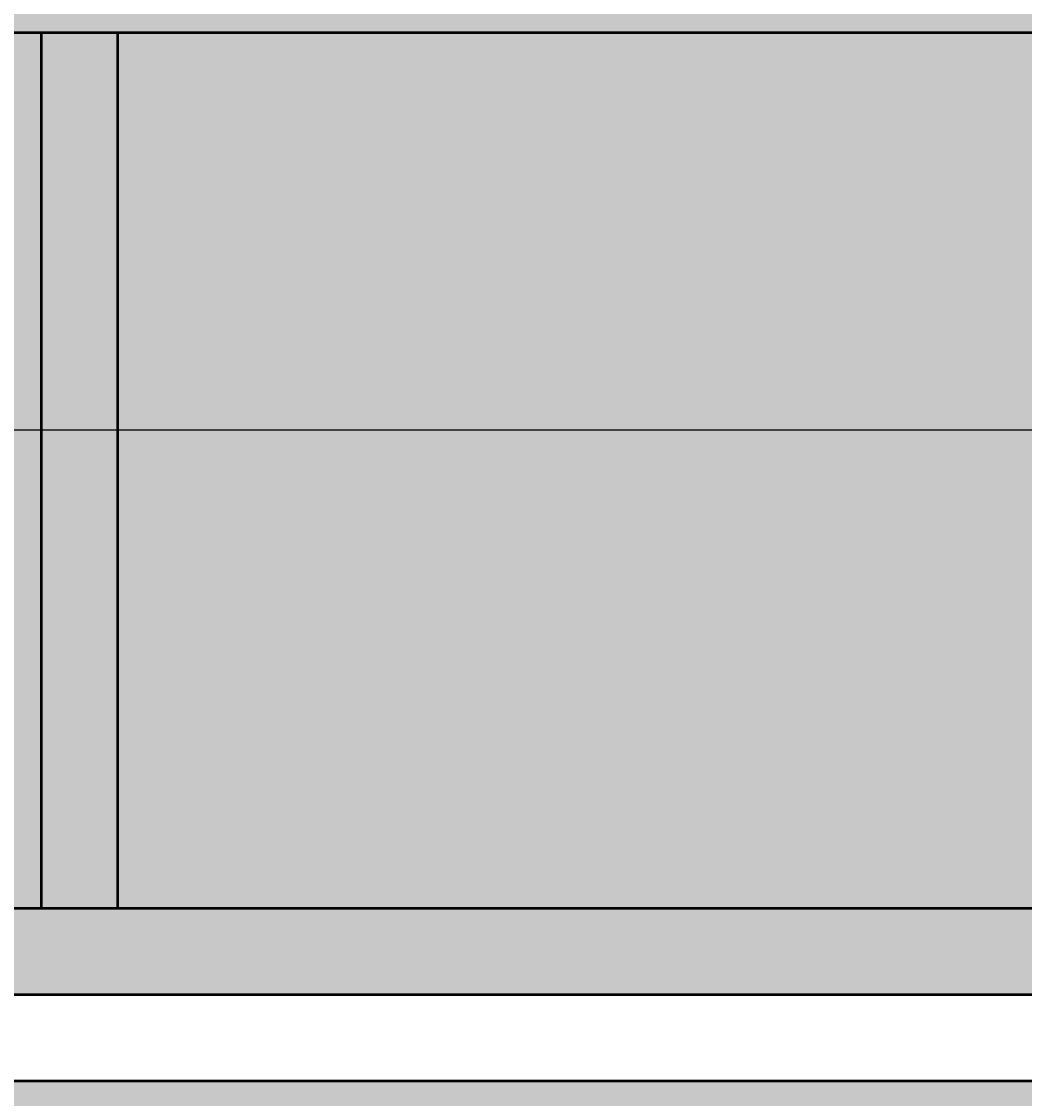
# Model space of a CAD drawing. Units: inches. Extents: x -12 to 334, y -10 to 186.
# Tile 38 of 77: x 129 to 152, y 65 to 90. Entities that reach past the tile are written whole.
import ezdxf

# ---------------------------------------------------------------- set-up
doc = ezdxf.new("R2010")
doc.units = ezdxf.units.IN
doc.header["$MEASUREMENT"] = 0
for name, color, linetype, lineweight in [('M-DIMS', 2, 'Continuous', 18), ('M-EQPM', 7, 'Continuous', 50), ('M-EQPM-PATT', 8, 'Continuous', 18)]:
    doc.layers.add(name, color=color, linetype=linetype, lineweight=lineweight)
doc.styles.get("Standard").update_dxf_attribs({"font": 'arial.ttf'})
doc.dimstyles.get("Standard").update_dxf_attribs({"dimtxt": 0.18, "dimasz": 0.18, "dimexe": 0.18, "dimexo": 0.0625, "dimgap": 0.09, "dimtad": 0, "dimtih": 1, "dimtoh": 1, "dimdec": 4, "dimzin": 0, "dimdsep": 46, "dimtxsty": 'Standard', "dimcen": 0.09, "dimadec": 0, "dimazin": 0, "dimtfac": 1, "dimtdec": 4, "dimtofl": 0, "dimtmove": 0, "dimatfit": 3, "dimfxl": 1, "dimtolj": 1, "dimtzin": 0, "dimarcsym": 0})

# ---------------------------------------------------------------- blocks, each defined once
blk = doc.blocks.new('*D1')
at = {"layer": 'Defpoints', "color": 0, "transparency": 16777216}
for p in [(281.426, 91.899), (3.376, 80.692), (281.426, 14.304)]:
    blk.add_point(p, dxfattribs=at)
at = {"layer": 'M-DIMS', "color": 0, "lineweight": -2, "transparency": 16777216}
for p, q in [((281.426, 91.836), (281.426, 14.124)), ((3.376, 80.629), (3.376, 14.124)), ((3.556, 14.304), (141.935, 14.304)), ((281.246, 14.304), (142.867, 14.304))]:
    blk.add_line(p, q, dxfattribs=at)
at = {"layer": 'M-DIMS', "color": 0, "transparency": 16777216}
for points in [[(3.556, 14.334), (3.556, 14.274), (3.376, 14.304)], [(281.246, 14.334), (281.246, 14.274), (281.426, 14.304)]]:
    blk.add_solid(points, dxfattribs=at)
at = {"layer": 'M-DIMS', "color": 0, "transparency": 16777216, "insert": (142.401, 14.304), "char_height": 0.18, "attachment_point": 5}
blk.add_mtext('\\A1;278.05', dxfattribs=at)
blk = doc.blocks.new('*D17')
at = {"layer": 'Defpoints', "color": 0, "transparency": 16777216}
for p in [(106.177, 102.896), (105.892, 56.321), (295.976, 56.321)]:
    blk.add_point(p, dxfattribs=at)
at = {"layer": 'M-DIMS', "color": 0, "lineweight": -2, "transparency": 16777216}
for p, q in [((106.24, 102.896), (296.156, 102.896)), ((295.976, 102.716), (295.976, 79.79)), ((295.976, 56.501), (295.976, 79.426)), ((105.954, 56.321), (296.156, 56.321))]:
    blk.add_line(p, q, dxfattribs=at)
at = {"layer": 'M-DIMS', "color": 0, "transparency": 16777216}
for points in [[(295.946, 102.716), (296.006, 102.716), (295.976, 102.896)], [(295.946, 56.501), (296.006, 56.501), (295.976, 56.321)]]:
    blk.add_solid(points, dxfattribs=at)
at = {"layer": 'M-DIMS', "color": 0, "transparency": 16777216, "insert": (295.976, 79.608), "char_height": 0.18, "attachment_point": 5}
blk.add_mtext('\\A1;46.575', dxfattribs=at)
blk = doc.blocks.new('*D35')
at = {"layer": 'Defpoints', "color": 0, "transparency": 16777216}
for p in [(216.428, 98.108), (-11.174, 61.105), (216.428, 61.105)]:
    blk.add_point(p, dxfattribs=at)
at = {"layer": 'M-DIMS', "color": 0, "lineweight": -2, "transparency": 16777216}
for p, q in [((216.365, 98.108), (-11.354, 98.108)), ((-11.174, 97.928), (-11.174, 79.788)), ((-11.174, 61.285), (-11.174, 79.424)), ((216.365, 61.105), (-11.354, 61.105))]:
    blk.add_line(p, q, dxfattribs=at)
at = {"layer": 'M-DIMS', "color": 0, "transparency": 16777216}
for points in [[(-11.204, 97.928), (-11.144, 97.928), (-11.174, 98.108)], [(-11.204, 61.285), (-11.144, 61.285), (-11.174, 61.105)]]:
    blk.add_solid(points, dxfattribs=at)
at = {"layer": 'M-DIMS', "color": 0, "transparency": 16777216, "insert": (-11.174, 79.606), "char_height": 0.18, "attachment_point": 5}
blk.add_mtext('\\A1;37', dxfattribs=at)
blk = doc.blocks.new('*D39')
at = {"layer": 'Defpoints', "color": 0, "transparency": 16777216}
for p in [(279.726, 80.692), (-11.174, 45.854), (269.381, 45.854)]:
    blk.add_point(p, dxfattribs=at)
at = {"layer": 'M-DIMS', "color": 0, "lineweight": -2, "transparency": 16777216}
for p, q in [((279.664, 80.692), (-11.354, 80.692)), ((-11.174, 80.512), (-11.174, 63.455)), ((-11.174, 46.034), (-11.174, 63.091)), ((269.318, 45.854), (-11.354, 45.854))]:
    blk.add_line(p, q, dxfattribs=at)
at = {"layer": 'M-DIMS', "color": 0, "transparency": 16777216}
for points in [[(-11.204, 80.512), (-11.144, 80.512), (-11.174, 80.692)], [(-11.204, 46.034), (-11.144, 46.034), (-11.174, 45.854)]]:
    blk.add_solid(points, dxfattribs=at)
at = {"layer": 'M-DIMS', "color": 0, "transparency": 16777216, "insert": (-11.174, 63.273), "char_height": 0.18, "attachment_point": 5}
blk.add_mtext('\\A1;34.84', dxfattribs=at)

msp = doc.modelspace()

# ---------------------------------------------------------------- hatches: boundary and pattern name
at = {"layer": 'M-EQPM-PATT'}
h = msp.add_hatch(color=256, dxfattribs=at)
h.set_gradient(color1=(205, 32, 39), color2=(205, 32, 39), tint=1)
h.paths.add_polyline_path([(64.5, 80.754), (64.5, 89.8963), (226.6083, 89.8963, -1), (226.6083, 69.6117), (64.5, 69.6117), (64.5, 78.754), (4.4744, 78.754, 0.384914), (23.5807, 61.4872), (37.1002, 61.4872), (37.1002, 33.6752), (53.1002, 33.6752), (53.1002, 61.4872), (64.5, 61.4872), (64.5, 63.6117), (226.6083, 63.6117, 1), (226.6083, 95.8963), (64.5, 95.8963), (64.5, 99.8958), (53.1002, 99.8958), (53.1002, 127.7078), (37.1002, 127.7078), (37.1002, 99.8958), (23.5807, 99.8958, 0.4132606), (4.3766, 80.754)])
h.paths.add_polyline_path([(64.5, 91.8963), (64.5, 93.8963), (226.6083, 93.8963, -1), (226.6083, 65.6117), (64.5, 65.6117), (64.5, 67.6117), (226.6083, 67.6117, 1), (226.6083, 91.8963)], flags=16)
h = msp.add_hatch(color=256, dxfattribs=at)
h.set_gradient(color1=(99, 100, 102), color2=(99, 100, 102), tint=1)
h.paths.add_polyline_path([(72.9244, 95.8963), (75.9244, 95.8963), (75.9244, 109.0583), (72.9244, 109.0583)])
h.paths.add_polyline_path([(72.9244, 50.4497), (75.9244, 50.4497), (75.9244, 63.6117), (72.9244, 63.6117)])
h.paths.add_polyline_path([(75.9244, 91.8963), (75.9244, 93.8963), (72.9244, 93.8963), (72.9244, 91.8963)])
h.paths.add_polyline_path([(75.9244, 65.6117), (75.9244, 67.6117), (72.9244, 67.6117), (72.9244, 65.6117)])
h.paths.add_polyline_path([(129.093, 69.6117), (130.8573, 69.6117), (130.8573, 89.8963), (129.093, 89.8963)])
h.paths.add_polyline_path([(129.093, 98.1081), (129.093, 95.8963), (130.8573, 95.8963), (130.8573, 98.1081)])
h.paths.add_polyline_path([(130.8573, 61.1045), (130.8573, 63.6117), (129.093, 63.6117), (129.093, 61.1045)])
h.paths.add_polyline_path([(170.9079, 69.6117), (172.6722, 69.6117), (172.6722, 89.8963), (170.9079, 89.8963)])
h.paths.add_polyline_path([(172.6722, 95.8963), (172.6722, 98.1081), (170.9079, 98.1081), (170.9079, 95.8963)])
h.paths.add_polyline_path([(170.9079, 61.1045), (172.6722, 61.1045), (172.6722, 63.6117), (170.9079, 63.6117)])
h.paths.add_polyline_path([(218.1922, 63.6117), (216.4278, 63.6117), (216.4278, 61.1045), (218.1922, 61.1045)])
h.paths.add_polyline_path([(216.4278, 69.6117), (218.1922, 69.6117), (218.1922, 89.8963), (216.4278, 89.8963)])
h.paths.add_polyline_path([(216.4278, 95.8963), (218.1922, 95.8963), (218.1922, 98.1081), (216.4278, 98.1081)])
h = msp.add_hatch(color=256, dxfattribs=at)
h.set_gradient(color1=(94, 103, 175), color2=(94, 103, 175), tint=1)
h.paths.add_polyline_path([(129.093, 89.8963), (86.8879, 89.8963), (86.8879, 69.6117), (129.093, 69.6117)], flags=17)
h.paths.add_polyline_path([(170.9079, 89.8963), (130.8573, 89.8963), (130.8573, 69.6117), (170.9079, 69.6117)], flags=17)
h.paths.add_polyline_path([(216.4278, 89.8963), (172.6722, 89.8963), (172.6722, 69.6117), (216.4278, 69.6117)], flags=17)
h.paths.add_polyline_path([(245.9354, 82.6969), (247.9354, 82.6969), (247.9354, 46.8541), (268.3808, 46.8541, 0.0998398), (279.7263, 80.6915), (251.9801, 80.6915, 0.4142136), (231.7758, 100.8958), (84.7229, 100.8958), (84.7229, 109.0583), (83.7229, 109.0583), (83.7229, 95.8963), (129.093, 95.8963), (129.093, 98.1081), (130.8573, 98.1081), (130.8573, 95.8963), (170.9079, 95.8963), (170.9079, 98.1081), (172.6722, 98.1081), (172.6722, 95.8963), (216.4278, 95.8963), (216.4278, 98.1081), (218.1922, 98.1081), (218.1922, 95.8963), (226.6083, 95.8963, -1), (226.6083, 63.6117), (218.1922, 63.6117), (218.1922, 61.1045), (216.4278, 61.1045), (216.4278, 63.6117), (172.6722, 63.6117), (172.6722, 61.1045), (170.9079, 61.1045), (170.9079, 63.6117), (130.8573, 63.6117), (130.8573, 61.1045), (129.093, 61.1045), (129.093, 63.6117), (87.8879, 63.6117), (87.8879, 56.3205), (105.8919, 56.3205), (105.8919, 28.8541), (115.8919, 28.8541), (115.8919, 46.8541), (222.5761, 46.8541), (222.5761, 30.8541), (232.5761, 30.8541), (232.5761, 46.8541), (245.9354, 46.8541)])
h.paths.add_polyline_path([(86.8879, 89.8963), (75.9244, 89.8963), (75.9244, 69.6117), (86.8879, 69.6117)])
h.paths.add_polyline_path([(83.7229, 109.0583), (75.9244, 109.0583), (75.9244, 95.8963), (83.7229, 95.8963)])
h.paths.add_polyline_path([(226.6083, 89.8963), (218.1922, 89.8963), (218.1922, 69.6117), (226.6083, 69.6117, 1)], flags=17)

# ---------------------------------------------------------------- linework, layer by layer
at = {"layer": 'M-EQPM'}
for points in [[(64.5, 65.6117), (226.6083, 65.6117, 1), (226.6083, 93.8963), (64.5, 93.8963)], [(64.5, 67.6117), (226.6083, 67.6117, 1), (226.6083, 91.8963), (64.5, 91.8963)], [(64.5, 69.6117), (226.6083, 69.6117, 1), (226.6083, 89.8963), (64.5, 89.8963)]]:
    msp.add_lwpolyline(points, format="xyb", dxfattribs=at)
for points in [[(129.093, 69.6117), (129.093, 89.8963)], [(130.8573, 89.8963), (130.8573, 69.6117)]]:
    msp.add_lwpolyline(points, dxfattribs=at)

# ---------------------------------------------------------------- dimensions: what is measured, and where the dimension line sits
at = {"layer": 'M-DIMS'}
for base, p1, p2, override, picture, middle in [((295.9756, 56.3205), (106.1771, 102.8958), (105.8919, 56.3205), {"dimdec": 3, "dimlfac": 1, "dimrnd": 0, "dimzin": 0, "dimdsep": 46, "dimlunit": 2}, '*D17', (295.9756, 79.6082)), ((-11.1736, 61.1045), (216.4278, 98.1081), (216.4278, 61.1045), {"dimdec": 0, "dimlfac": 1, "dimrnd": 0, "dimzin": 0, "dimdsep": 46, "dimlunit": 2}, '*D35', (-11.1735, 79.6063)), ((-11.1736, 45.8541), (279.7263, 80.6915), (269.3808, 45.8541), {"dimdec": 2, "dimlfac": 1, "dimrnd": 0, "dimzin": 0, "dimdsep": 46, "dimlunit": 2}, '*D39', (-11.1735, 63.2728))]:
    dim = msp.add_linear_dim(base=base, p1=p1, p2=p2, angle=90, dimstyle='Standard', override=override, dxfattribs=at)
    dim.commit()
    dim.dimension.update_dxf_attribs({"geometry": picture, "text_midpoint": middle})
dim = msp.add_linear_dim(base=(281.4256, 14.3041), p1=(3.3765, 80.6915), p2=(281.4256, 91.8988), dimstyle='Standard', override={"dimdec": 2, "dimlfac": 1, "dimrnd": 0, "dimzin": 0, "dimdsep": 46, "dimlunit": 2}, dxfattribs=at)
dim.commit()
dim.dimension.update_dxf_attribs({"geometry": '*D1', "text_midpoint": (142.401, 14.3041)})

doc.saveas('drawing.dxf')
